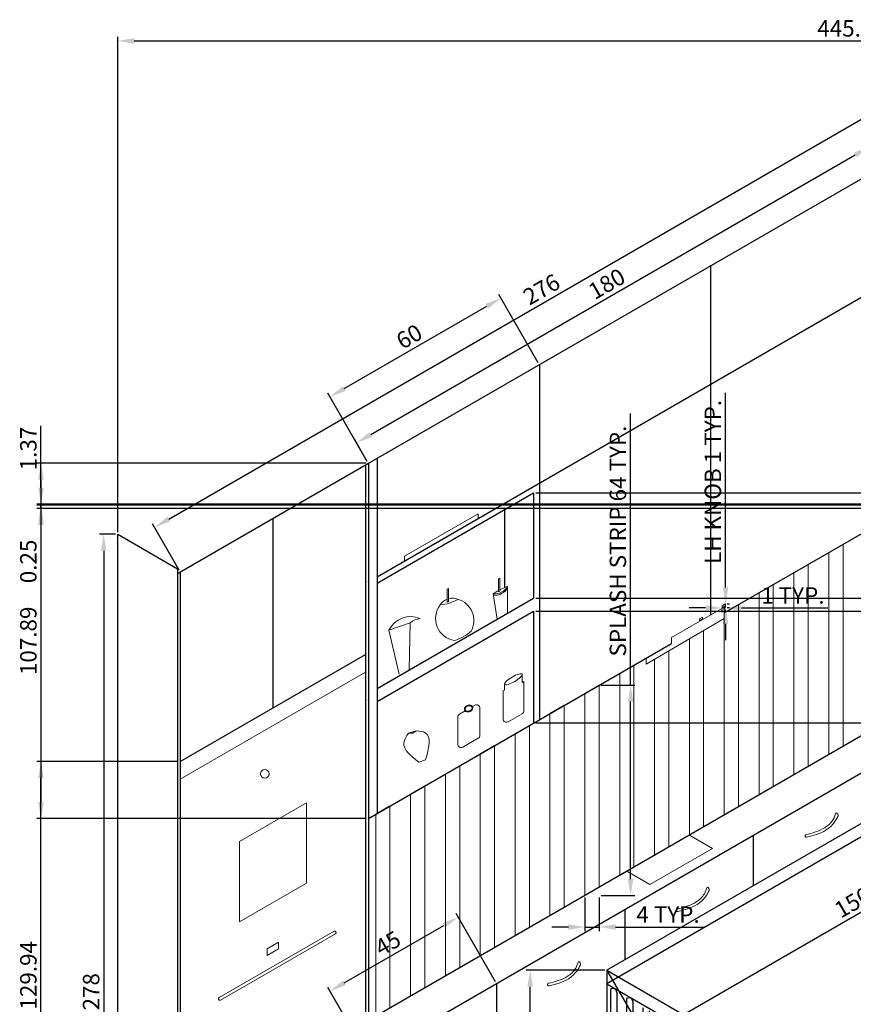
# Model space of a CAD drawing. Units: centimetres. Extents: x 2148 to 2649, y 4226 to 4785.
# Tile 2 of 6: x 2148 to 2402, y 4445 to 4744. Entities that reach past the tile are written whole.
import ezdxf

# ---------------------------------------------------------------- set-up
doc = ezdxf.new("R2010")
doc.units = ezdxf.units.CM
for name, color, linetype, lineweight in [('A-ANNO-DIMS', 63, 'Continuous', 18), ('A-ANNO-REFR', 8, 'Continuous', 13), ('A-EQPM', 30, 'Continuous', 18), ('A-FLOR-BSPL', 21, 'Continuous', 13), ('A-FLOR-CASE', 21, 'Continuous', 25), ('A-FLOR-CASE-HDW', 21, 'Continuous', 18), ('A-FLOR-CASE-TALL', 30, 'Continuous', 30), ('A-FLOR-CTOP', 21, 'Continuous', 25), ('A-FURN-ACCS', 21, 'Continuous', 13), ('TABLE', 30, 'Continuous', 25)]:
    doc.layers.add(name, color=color, linetype=linetype, lineweight=lineweight)
doc.styles.get("Standard").update_dxf_attribs({"font": 'arial.ttf'})
doc.dimstyles.new('ISO-25', dxfattribs={"dimtxt": 5, "dimasz": 5, "dimexe": 1.25, "dimexo": 0.625, "dimtad": 1, "dimdec": 1, "dimtxsty": 'Standard', "dimcen": 2.5, "dimadec": 0, "dimazin": 0, "dimtfac": 1, "dimtdec": 1, "dimtmove": 0, "dimatfit": 3, "dimfxl": 1, "dimarcsym": 0})

# ---------------------------------------------------------------- blocks, each defined once
blk = doc.blocks.new('*D1')
at = {"layer": 'A-ANNO-DIMS', "color": 0, "lineweight": -2, "transparency": 16777216}
for p, q in [((2409.99, 4699.79), (2406.08, 4706.55)), ((2255.15, 4617.96), (2402.38, 4702.96)), ((2254.1, 4609.79), (2250.2, 4616.55))]:
    blk.add_line(p, q, dxfattribs=at)
at = {"layer": 'A-ANNO-DIMS', "color": 0, "transparency": 16777216}
for points in [[(2401.96, 4703.69), (2402.8, 4702.24), (2406.71, 4705.46)], [(2254.74, 4618.69), (2255.57, 4617.24), (2250.82, 4615.46)]]:
    blk.add_solid(points, dxfattribs=at)
at = {"layer": 'Defpoints', "color": 0, "transparency": 16777216}
for p in [(2406.71, 4705.46), (2410.3, 4699.24), (2254.42, 4609.24)]:
    blk.add_point(p, dxfattribs=at)
at = {"layer": 'A-ANNO-DIMS', "color": 0, "transparency": 16777216, "insert": (2327.18, 4663.22), "char_height": 5, "attachment_point": 5, "rotation": 30}
blk.add_mtext('180', dxfattribs=at)
blk = doc.blocks.new('RECTANGLE')
for p, q in [((2256.66, 4502.65), (2260.99, 4505.15)), ((2256.66, 4502.65), (2256.66, 4441.26)), ((2260.99, 4443.76), (2260.99, 4505.15)), ((2256.66, 4441.26), (2260.99, 4443.76))]:
    blk.add_line(p, q)
blk = doc.blocks.new('*D4')
at = {"layer": 'A-ANNO-DIMS', "color": 0, "lineweight": -2, "transparency": 16777216}
for p, q in [((2177.63, 4587.69), (2172.75, 4587.69)), ((2174, 4582.69), (2174, 4314.69)), ((2177.63, 4309.69), (2172.75, 4309.69))]:
    blk.add_line(p, q, dxfattribs=at)
at = {"layer": 'A-ANNO-DIMS', "color": 0, "transparency": 16777216}
for points in [[(2173.16, 4582.69), (2174.83, 4582.69), (2174, 4587.69)], [(2173.16, 4314.69), (2174.83, 4314.69), (2174, 4309.69)]]:
    blk.add_solid(points, dxfattribs=at)
at = {"layer": 'Defpoints', "color": 0, "transparency": 16777216}
for p in [(2178.26, 4587.69), (2174, 4309.69), (2178.26, 4309.69)]:
    blk.add_point(p, dxfattribs=at)
at = {"layer": 'A-ANNO-DIMS', "color": 0, "transparency": 16777216, "insert": (2170.82, 4448.69), "char_height": 5, "attachment_point": 5, "rotation": 90}
blk.add_mtext('278', dxfattribs=at)
blk = doc.blocks.new('*D5')
at = {"layer": 'A-ANNO-DIMS', "color": 0, "lineweight": -2, "transparency": 16777216}
for p, q in [((2435.97, 4714.79), (2427.84, 4728.87)), ((2193.77, 4592.29), (2424.13, 4725.29)), ((2196.95, 4576.79), (2188.81, 4590.87))]:
    blk.add_line(p, q, dxfattribs=at)
at = {"layer": 'A-ANNO-DIMS', "color": 0, "transparency": 16777216}
for points in [[(2423.72, 4726.01), (2424.55, 4724.57), (2428.46, 4727.79)], [(2193.35, 4593.01), (2194.19, 4591.57), (2189.44, 4589.79)]]:
    blk.add_solid(points, dxfattribs=at)
at = {"layer": 'Defpoints', "color": 0, "transparency": 16777216}
for p in [(2428.46, 4727.79), (2436.28, 4714.24), (2197.26, 4576.24)]:
    blk.add_point(p, dxfattribs=at)
at = {"layer": 'A-ANNO-DIMS', "color": 0, "transparency": 16777216, "insert": (2307.36, 4661.54), "char_height": 5, "attachment_point": 5, "rotation": 30}
blk.add_mtext('276', dxfattribs=at)
blk = doc.blocks.new('T')
for p, q in [((2448.14, 4353.09), (2318.24, 4278.09)), ((2522.91, 4309.92), (2448.14, 4353.09)), ((2403.01, 4232.03), (2522.91, 4301.26)), ((2318.24, 4278.09), (2398.01, 4232.03))]:
    blk.add_line(p, q)
for centre, start, end in [((2520.41, 4305.59), 300, 60), ((2400.51, 4236.36), 240, 300)]:
    blk.add_arc(centre, 5, start, end)
blk = doc.blocks.new('FRUITS')
for centre in [(2416.61, 4474.09), (2427.91, 4474), (2437.55, 4475.46), (2421.39, 4472.47)]:
    blk.add_circle(centre, 1.88)
for centre, start, end in [((2425.68, 4477.15), 250.6785, 228.1131), ((2431.37, 4476.49), 347.1742, 260.6235), ((2420.14, 4474.94), 339.5983, 177.9649), ((2423.8, 4473.97), 252.9307, 170.9248), ((2432.9, 4474.21), 301.9934, 262.6603), ((2420.14, 4474.94), 208.8656, 254.0869)]:
    blk.add_arc(centre, 1.88, start, end)
for start_param, end_param in [(5.976427, 9.8373), (4.471607, 4.914134)]:
    blk.add_ellipse((2418.08, 4470.84), major_axis=(-2.82, 1), ratio=0.809593, start_param=start_param, end_param=end_param)
for points, knots in [([(2406.43, 4471.88), (2412.49, 4474.08), (2424.62, 4478.48), (2437.33, 4476.24), (2443.7, 4475.12)], [0, 0, 0, 0, 18.967698, 37.99902, 37.99902, 37.99902, 37.99902]), ([(2406.43, 4471.88), (2409.22, 4465.94), (2414.78, 4454.12), (2438.7, 4455.69), (2442.02, 4468.59), (2443.7, 4475.12)], [0, 0, 0, 0, 18.249558, 36.298645, 54.808813, 54.808813, 54.808813, 54.808813]), ([(2406.43, 4471.88), (2411.36, 4471.29), (2423.93, 4469.77), (2436.23, 4473.1), (2443.7, 4475.12)], [0, 0, 0, 0, 14.783083, 37.710843, 37.710843, 37.710843, 37.710843])]:
    blk.add_open_spline(points, degree=3, knots=knots)
blk = doc.blocks.new('TABLE 3')
for p, q in [((2534.09, 4482.72), (2534.09, 4425.1)), ((2529.29, 4472.97), (2529.29, 4424.6)), ((2531.69, 4473.13), (2531.69, 4424.8)), ((2531.69, 4473.13), (2531.69, 4424.8)), ((2523.55, 4469.66), (2523.55, 4424.61)), ((2525.96, 4471.05), (2525.96, 4423.89)), ((2525.96, 4469.82), (2525.96, 4423.89)), ((2529.29, 4471.74), (2529.29, 4424.6)), ((2520.23, 4467.74), (2520.23, 4430.04)), ((2520.23, 4466.51), (2520.23, 4430.04)), ((2523.55, 4468.43), (2523.55, 4424.61)), ((2514.5, 4464.43), (2514.5, 4434.64)), ((2517.82, 4466.35), (2517.82, 4432.4)), ((2517.82, 4465.12), (2517.82, 4432.4)), ((2508.76, 4461.12), (2508.76, 4432.32)), ((2512.09, 4463.04), (2512.09, 4434.39)), ((2512.09, 4461.81), (2512.09, 4434.39)), ((2514.5, 4463.2), (2514.5, 4434.64)), ((2503.03, 4457.81), (2503.03, 4427.36)), ((2506.35, 4459.73), (2506.35, 4430.48)), ((2506.35, 4458.5), (2506.35, 4430.48)), ((2326.91, 4455.22), (2326.91, 4314.1)), ((2497.3, 4454.5), (2497.3, 4419.33)), ((2500.62, 4456.42), (2500.62, 4424.52)), ((2500.62, 4455.19), (2500.62, 4424.52)), ((2503.03, 4456.58), (2503.03, 4427.36)), ((2494.89, 4453.11), (2494.89, 4413.65)), ((2494.89, 4451.88), (2494.89, 4413.65)), ((2497.3, 4453.27), (2497.3, 4419.33)), ((2328.01, 4449.42), (2328.01, 4314.3)), ((2329.93, 4448.55), (2329.93, 4313.58)), ((2489.16, 4449.8), (2489.16, 4412.9)), ((2489.16, 4448.57), (2489.16, 4412.9)), ((2491.57, 4451.19), (2491.57, 4413.39)), ((2491.57, 4449.96), (2491.57, 4413.39)), ((2332.9, 4446.6), (2332.9, 4311.48)), ((2334.82, 4445.73), (2334.82, 4310.75)), ((2483.42, 4446.49), (2483.42, 4412.26)), ((2485.83, 4447.88), (2485.83, 4412.44)), ((2485.83, 4446.65), (2485.83, 4412.44)), ((2337.79, 4443.77), (2337.79, 4308.66)), ((2339.71, 4442.9), (2339.71, 4307.93)), ((2480.1, 4443.34), (2480.1, 4410.27)), ((2480.1, 4443.34), (2480.1, 4410.27)), ((2483.42, 4445.26), (2483.42, 4412.26)), ((2342.68, 4440.95), (2342.68, 4305.83)), ((2344.61, 4440.08), (2344.61, 4305.11)), ((2474.37, 4440.03), (2474.37, 4418.94)), ((2477.69, 4441.95), (2477.69, 4415.46)), ((2477.69, 4441.95), (2477.69, 4415.46)), ((2347.58, 4438.12), (2347.58, 4303.01)), ((2349.5, 4437.25), (2349.5, 4302.28)), ((2468.64, 4436.72), (2468.64, 4419.49)), ((2468.64, 4436.72), (2468.64, 4419.49)), ((2352.47, 4435.3), (2352.47, 4300.18)), ((2354.39, 4434.43), (2354.39, 4299.46)), ((2466.23, 4435.33), (2466.23, 4418.06)), ((2466.23, 4435.33), (2466.23, 4418.06)), ((2357.36, 4432.47), (2357.36, 4297.36)), ((2359.28, 4431.6), (2359.28, 4296.63)), ((2460.49, 4432.02), (2460.49, 4413.4)), ((2460.49, 4432.02), (2460.49, 4413.4)), ((2462.9, 4433.41), (2462.9, 4415.61)), ((2462.9, 4433.41), (2462.9, 4415.61)), ((2362.25, 4429.65), (2362.25, 4294.53)), ((2364.18, 4428.78), (2364.18, 4293.81)), ((2454.76, 4428.71), (2454.76, 4405.82)), ((2457.17, 4430.1), (2457.17, 4409.54)), ((2457.17, 4430.1), (2457.17, 4409.54)), ((2367.15, 4426.82), (2367.15, 4291.71)), ((2369.07, 4425.95), (2369.07, 4290.98)), ((2449.03, 4425.4), (2449.03, 4290.41)), ((2451.44, 4426.79), (2451.44, 4291.8)), ((2372.04, 4424), (2372.04, 4288.88)), ((2373.96, 4423.13), (2373.96, 4288.16)), ((2443.3, 4422.09), (2443.3, 4287.1)), ((2445.7, 4423.48), (2445.7, 4288.49)), ((2376.93, 4421.17), (2376.93, 4286.06)), ((2378.85, 4420.3), (2378.85, 4285.33)), ((2437.56, 4418.78), (2437.56, 4283.79)), ((2439.97, 4420.17), (2439.97, 4285.18)), ((2381.82, 4418.35), (2381.82, 4283.23)), ((2383.75, 4417.48), (2383.75, 4282.51)), ((2434.24, 4416.86), (2434.24, 4281.87)), ((2386.72, 4415.52), (2386.72, 4280.41)), ((2388.64, 4414.65), (2388.64, 4279.68)), ((2391.61, 4412.7), (2391.61, 4277.58)), ((2428.51, 4413.55), (2428.51, 4278.56)), ((2431.83, 4415.47), (2431.83, 4280.48)), ((2393.53, 4411.83), (2393.53, 4276.86)), ((2396.5, 4409.88), (2396.5, 4274.76)), ((2422.77, 4410.24), (2422.77, 4275.25)), ((2426.1, 4412.16), (2426.1, 4277.17)), ((2398.42, 4409.01), (2398.42, 4274.03)), ((2400.52, 4408.63), (2400.52, 4271.6)), ((2417.84, 4408.63), (2417.84, 4271.6)), ((2420.37, 4408.85), (2420.37, 4273.86)), ((2460.49, 4392.27), (2460.49, 4323.14)), ((2503.03, 4391.9), (2503.03, 4330.42)), ((2462.9, 4390.64), (2462.9, 4321.75)), ((2500.62, 4390.56), (2500.62, 4329.03)), ((2512.09, 4390.5), (2512.09, 4334.07)), ((2523.55, 4388.81), (2523.55, 4340.69)), ((2525.96, 4389.23), (2525.96, 4342.08)), ((2534.09, 4391.22), (2534.09, 4381.5)), ((2466.23, 4388.14), (2466.23, 4319.83)), ((2468.64, 4386.14), (2468.64, 4318.44)), ((2491.57, 4386.54), (2491.57, 4323.8)), ((2494.89, 4387.83), (2494.89, 4325.72)), ((2520.23, 4388.33), (2520.23, 4338.77)), ((2477.69, 4383.14), (2477.69, 4315.79)), ((2480.1, 4383.51), (2480.1, 4317.18)), ((2483.42, 4384.17), (2483.42, 4319.1)), ((2485.83, 4384.76), (2485.83, 4320.49)), ((2534.09, 4384.82), (2534.09, 4341.83)), ((2529.29, 4341), (2529.29, 4336.74)), ((2525.96, 4339.08), (2525.96, 4334.83)), ((2518.06, 4329.46), (2529.88, 4336.29)), ((2520.23, 4335.77), (2520.23, 4331.52)), ((2523.55, 4337.69), (2523.55, 4333.43)), ((2512.09, 4331.07), (2512.09, 4326.82)), ((2508.53, 4323.96), (2515.55, 4328.01)), ((2500.62, 4323.12), (2500.62, 4322.24)), ((2503.03, 4324.51), (2503.03, 4321.59)), ((2494.89, 4319.81), (2494.89, 4316.89)), ((2503.09, 4320.82), (2506.45, 4322.76)), ((2460.49, 4317.23), (2460.49, 4297.03)), ((2475.33, 4304.79), (2496.19, 4316.83)), ((2491.57, 4317.89), (2491.57, 4314.97)), ((2498.19, 4317.99), (2500.49, 4319.32)), ((2326.91, 4314.1), (2406.68, 4268.04)), ((2462.9, 4315.84), (2462.9, 4298.42)), ((2466.23, 4313.92), (2466.23, 4300.34)), ((2485.83, 4314.58), (2485.83, 4311.66)), ((2489.16, 4316.5), (2489.16, 4313.58)), ((2468.64, 4312.53), (2468.64, 4301.73)), ((2480.1, 4311.27), (2480.1, 4308.35)), ((2483.42, 4313.19), (2483.42, 4310.27)), ((2477.69, 4309.88), (2477.69, 4306.96)), ((2455.96, 4293.61), (2473.25, 4303.59)), ((2411.68, 4268.04), (2454.39, 4292.7))]:
    blk.add_line(p, q)
for centre, radius, start, end in [((2530.67, 4472.12), 1.44, 44.5272, 195.4728), ((2524.94, 4468.81), 1.44, 44.5272, 195.4728), ((2519.2, 4465.5), 1.44, 44.5272, 195.4728), ((2513.47, 4462.19), 1.44, 44.5272, 195.4728), ((2507.74, 4458.88), 1.44, 44.5272, 195.4728), ((2502.01, 4455.57), 1.44, 44.5272, 195.4728), ((2496.27, 4452.26), 1.44, 44.5272, 195.4728), ((2490.54, 4448.95), 1.44, 44.5272, 195.4728), ((2484.81, 4445.64), 1.44, 44.5272, 195.4728), ((2479.08, 4442.33), 1.44, 44.5272, 195.4728), ((2473.34, 4439.02), 1.44, 44.5272, 195.4728), ((2467.61, 4435.71), 1.44, 44.5272, 195.4728), ((2461.88, 4432.4), 1.44, 44.5272, 195.4728), ((2456.15, 4429.09), 1.44, 44.5272, 195.4728), ((2450.41, 4425.78), 1.44, 44.5272, 195.4728), ((2444.68, 4422.47), 1.44, 44.5272, 195.4728), ((2438.95, 4419.16), 1.44, 44.5272, 195.4728), ((2433.22, 4415.85), 1.44, 44.5272, 195.4728), ((2427.48, 4412.55), 1.44, 44.5272, 195.4728), ((2421.75, 4409.24), 1.44, 44.5272, 195.4728), ((2529.09, 4341.6), 5, 304.2234, 331.1295), ((2524.24, 4335.03), 1.74, 246.8122, 353.1878), ((2529.97, 4338.34), 1.74, 246.8122, 267.0744), ((2518.5, 4331.72), 1.74, 255.6127, 353.1878), ((2512.77, 4328.41), 1.74, 246.8122, 353.1878), ((2501.31, 4321.79), 1.74, 331.6217, 353.1878), ((2495.57, 4318.48), 1.74, 246.8122, 290.8785), ((2329.13, 4314.36), 1.12, 182.9367, 315.698), ((2489.84, 4315.17), 1.74, 246.8122, 353.1878), ((2334.02, 4311.54), 1.12, 182.9367, 315.698), ((2484.11, 4311.86), 1.74, 246.8122, 353.1878), ((2338.91, 4308.71), 1.12, 182.9367, 315.698), ((2478.38, 4308.55), 1.74, 246.8122, 353.1878), ((2343.8, 4305.89), 1.12, 182.9367, 315.698), ((2348.7, 4303.06), 1.12, 182.9367, 315.698), ((2353.59, 4300.24), 1.12, 182.9367, 315.698), ((2466.91, 4301.93), 1.74, 246.8122, 353.1878), ((2358.48, 4297.41), 1.12, 182.9367, 315.698), ((2461.18, 4298.62), 1.74, 246.8122, 353.1878), ((2363.37, 4294.59), 1.12, 182.9367, 315.698), ((2455.45, 4295.31), 1.74, 287.3713, 353.1878), ((2368.27, 4291.77), 1.12, 182.9367, 315.698), ((2449.71, 4292.01), 1.74, 246.8122, 353.1878), ((2373.16, 4288.94), 1.12, 182.9367, 315.698), ((2443.98, 4288.7), 1.74, 246.8122, 353.1878), ((2378.05, 4286.12), 1.12, 182.9367, 315.698), ((2438.25, 4285.39), 1.74, 246.8122, 353.1878), ((2382.94, 4283.29), 1.12, 182.9367, 315.698), ((2432.51, 4282.08), 1.74, 246.8122, 353.1878), ((2387.84, 4280.47), 1.12, 182.9367, 315.698), ((2426.78, 4278.77), 1.74, 246.8122, 353.1878), ((2392.73, 4277.64), 1.12, 182.9367, 315.698), ((2421.05, 4275.46), 1.74, 246.8122, 353.1878), ((2397.62, 4274.82), 1.12, 182.9367, 315.698), ((2409.18, 4272.37), 5, 240, 300)]:
    blk.add_arc(centre, radius, start, end)
for name, p in [('T', (8.67, 177.13)), ('T', (8.67, 173.04)), ('FRUITS', (0, 0))]:
    blk.add_blockref(name, p)
blk = doc.blocks.new('PULL-BASE-BOW')
for centre, radius, start, end in [((9.29, 6.64), 0.774, 341.702, 83.222), ((0.41, 0.41), 0.414, 116.0189, 282.6641)]:
    blk.add_arc(centre, radius, start, end)
for points, knots in [([(0.23, 0.79), (2.23, 1.29), (5.42, 2.1), (8.53, 4.9), (9.15, 6.73), (9.38, 7.41)], [0, 0, 0, 0, 6.127515, 9.756066, 11.887711, 11.887711, 11.887711, 11.887711]), ([(0.5, 0.01), (2.55, 0.54), (5.72, 1.35), (8.78, 4.08), (9.68, 5.75), (10.03, 6.4)], [0, 0, 0, 0, 6.234589, 9.67204, 11.894402, 11.894402, 11.894402, 11.894402])]:
    blk.add_open_spline(points, degree=3, knots=knots)
blk = doc.blocks.new('KNOB-ISO-L')
for p, q in [((0, 0.53), (0.92, 1.06)), ((0, 0), (0, 0.53)), ((0, 0), (0.92, 0.53)), ((0.92, 1.06), (0.92, 0.53))]:
    blk.add_line(p, q)
blk = doc.blocks.new('*D20')
at = {"layer": 'A-ANNO-DIMS', "color": 0, "lineweight": -2, "transparency": 16777216}
for p, q in [((2334.1, 4541.83), (2334.1, 4624.41)), ((2325.14, 4541.83), (2335.35, 4541.83)), ((2334.1, 4482.94), (2334.1, 4536.83)), ((2325.14, 4477.94), (2335.35, 4477.94))]:
    blk.add_line(p, q, dxfattribs=at)
at = {"layer": 'A-ANNO-DIMS', "color": 0, "transparency": 16777216}
for points in [[(2333.27, 4536.83), (2334.94, 4536.83), (2334.1, 4541.83)], [(2333.27, 4482.94), (2334.94, 4482.94), (2334.1, 4477.94)]]:
    blk.add_solid(points, dxfattribs=at)
at = {"layer": 'Defpoints', "color": 0, "transparency": 16777216}
for p in [(2324.52, 4541.83), (2334.1, 4541.83), (2324.52, 4477.94)]:
    blk.add_point(p, dxfattribs=at)
at = {"layer": 'A-ANNO-DIMS', "color": 0, "transparency": 16777216, "insert": (2330.89, 4585.62), "char_height": 5, "attachment_point": 5, "rotation": 90}
blk.add_mtext('SPLASH STRIP 64 TYP.', dxfattribs=at)
blk = doc.blocks.new('*D21')
at = {"layer": 'A-ANNO-DIMS', "color": 0, "lineweight": -2, "transparency": 16777216}
for p, q in [((2320.19, 4477.31), (2320.19, 4467.1)), ((2324.52, 4477.31), (2324.52, 4467.1)), ((2315.19, 4468.35), (2310.19, 4468.35)), ((2320.19, 4468.35), (2324.52, 4468.35)), ((2329.52, 4468.35), (2356.42, 4468.35))]:
    blk.add_line(p, q, dxfattribs=at)
at = {"layer": 'A-ANNO-DIMS', "color": 0, "transparency": 16777216}
for points in [[(2315.19, 4469.19), (2315.19, 4467.52), (2320.19, 4468.35)], [(2329.52, 4469.19), (2329.52, 4467.52), (2324.52, 4468.35)]]:
    blk.add_solid(points, dxfattribs=at)
at = {"layer": 'Defpoints', "color": 0, "transparency": 16777216}
for p in [(2320.19, 4477.94), (2324.52, 4477.94), (2324.52, 4468.35)]:
    blk.add_point(p, dxfattribs=at)
at = {"layer": 'A-ANNO-DIMS', "color": 0, "transparency": 16777216, "insert": (2345.47, 4471.48), "char_height": 5, "attachment_point": 5}
blk.add_mtext('4 TYP.', dxfattribs=at)
blk = doc.blocks.new('*D24')
at = {"layer": 'A-ANNO-DIMS', "color": 0, "lineweight": -2, "transparency": 16777216}
for p, q in [((2362.95, 4571.52), (2362.95, 4630.61)), ((2362.95, 4565.46), (2362.95, 4566.52)), ((2363.42, 4566.52), (2364.2, 4566.52)), ((2363.42, 4565.46), (2364.2, 4565.46)), ((2362.95, 4560.46), (2362.95, 4555.46))]:
    blk.add_line(p, q, dxfattribs=at)
at = {"layer": 'A-ANNO-DIMS', "color": 0, "transparency": 16777216}
for points in [[(2362.12, 4571.52), (2363.78, 4571.52), (2362.95, 4566.52)], [(2362.12, 4560.46), (2363.78, 4560.46), (2362.95, 4565.46)]]:
    blk.add_solid(points, dxfattribs=at)
at = {"layer": 'Defpoints', "color": 0, "transparency": 16777216}
for p in [(2362.79, 4566.52), (2362.79, 4565.46), (2362.95, 4566.52)]:
    blk.add_point(p, dxfattribs=at)
at = {"layer": 'A-ANNO-DIMS', "color": 0, "transparency": 16777216, "insert": (2359.74, 4603.57), "char_height": 5, "attachment_point": 5, "rotation": 90}
blk.add_mtext('LH KNOB 1 TYP.', dxfattribs=at)
blk = doc.blocks.new('*D25')
at = {"layer": 'A-ANNO-DIMS', "color": 0, "lineweight": -2, "transparency": 16777216}
for p, q in [((2356.87, 4565.3), (2351.87, 4565.3)), ((2361.87, 4565.3), (2362.79, 4565.3)), ((2367.79, 4565.3), (2394.02, 4565.3)), ((2361.87, 4564.84), (2361.87, 4564.05)), ((2362.79, 4564.84), (2362.79, 4564.05))]:
    blk.add_line(p, q, dxfattribs=at)
at = {"layer": 'A-ANNO-DIMS', "color": 0, "transparency": 16777216}
for points in [[(2356.87, 4566.13), (2356.87, 4564.47), (2361.87, 4565.3)], [(2367.79, 4566.13), (2367.79, 4564.47), (2362.79, 4565.3)]]:
    blk.add_solid(points, dxfattribs=at)
at = {"layer": 'Defpoints', "color": 0, "transparency": 16777216}
for p in [(2361.87, 4565.46), (2362.79, 4565.46), (2362.79, 4565.3)]:
    blk.add_point(p, dxfattribs=at)
at = {"layer": 'A-ANNO-DIMS', "color": 0, "transparency": 16777216, "insert": (2383.41, 4568.44), "char_height": 5, "attachment_point": 5}
blk.add_mtext('1 TYP.', dxfattribs=at)
blk = doc.blocks.new('*D40')
at = {"layer": 'A-ANNO-DIMS', "color": 0, "lineweight": -2, "transparency": 16777216}
for p, q in [((2306.06, 4639.79), (2294.09, 4660.53)), ((2247.08, 4631.94), (2290.38, 4656.94)), ((2254.1, 4609.79), (2242.13, 4630.53))]:
    blk.add_line(p, q, dxfattribs=at)
at = {"layer": 'A-ANNO-DIMS', "color": 0, "transparency": 16777216}
for points in [[(2289.97, 4657.67), (2290.8, 4656.22), (2294.71, 4659.44)], [(2246.67, 4632.67), (2247.5, 4631.22), (2242.75, 4629.44)]]:
    blk.add_solid(points, dxfattribs=at)
at = {"layer": 'Defpoints', "color": 0, "transparency": 16777216}
for p in [(2294.71, 4659.44), (2306.38, 4639.24), (2254.42, 4609.24)]:
    blk.add_point(p, dxfattribs=at)
at = {"layer": 'A-ANNO-DIMS', "color": 0, "transparency": 16777216, "insert": (2267.15, 4647.2), "char_height": 5, "attachment_point": 5, "rotation": 30}
blk.add_mtext('60', dxfattribs=at)
blk = doc.blocks.new('*D41')
at = {"layer": 'A-ANNO-DIMS', "color": 0, "lineweight": -2, "transparency": 16777216}
for p, q in [((2253.79, 4609.24), (2153.68, 4609.24)), ((2154.93, 4604.24), (2154.93, 4506.36)), ((2253.79, 4501.36), (2153.68, 4501.36))]:
    blk.add_line(p, q, dxfattribs=at)
at = {"layer": 'A-ANNO-DIMS', "color": 0, "transparency": 16777216}
for points in [[(2154.1, 4604.24), (2155.77, 4604.24), (2154.93, 4609.24)], [(2154.1, 4506.36), (2155.77, 4506.36), (2154.93, 4501.36)]]:
    blk.add_solid(points, dxfattribs=at)
at = {"layer": 'Defpoints', "color": 0, "transparency": 16777216}
for p in [(2254.42, 4609.24), (2154.93, 4501.36), (2254.42, 4501.36)]:
    blk.add_point(p, dxfattribs=at)
at = {"layer": 'A-ANNO-DIMS', "color": 0, "transparency": 16777216, "insert": (2151.75, 4555.3), "char_height": 5, "attachment_point": 5, "rotation": 90}
blk.add_mtext('107.89', dxfattribs=at)
blk = doc.blocks.new('*D42')
at = {"layer": 'A-ANNO-DIMS', "color": 0, "lineweight": -2, "transparency": 16777216}
for p, q in [((2305.27, 4600.28), (2648.78, 4600.28)), ((2647.53, 4595.28), (2647.53, 4573.32)), ((2305.27, 4568.32), (2648.78, 4568.32))]:
    blk.add_line(p, q, dxfattribs=at)
at = {"layer": 'A-ANNO-DIMS', "color": 0, "transparency": 16777216}
for points in [[(2646.7, 4595.28), (2648.37, 4595.28), (2647.53, 4600.28)], [(2646.7, 4573.32), (2648.37, 4573.32), (2647.53, 4568.32)]]:
    blk.add_solid(points, dxfattribs=at)
at = {"layer": 'Defpoints', "color": 0, "transparency": 16777216}
for p in [(2304.65, 4600.28), (2304.65, 4568.32), (2647.53, 4568.32)]:
    blk.add_point(p, dxfattribs=at)
at = {"layer": 'A-ANNO-DIMS', "color": 0, "transparency": 16777216, "insert": (2644.35, 4584.3), "char_height": 5, "attachment_point": 5, "rotation": 90}
blk.add_mtext('31.96', dxfattribs=at)
blk = doc.blocks.new('*D43')
at = {"layer": 'A-ANNO-DIMS', "color": 0, "lineweight": -2, "transparency": 16777216}
for p, q in [((2647.53, 4573.32), (2647.53, 4578.32)), ((2305.27, 4568.32), (2648.78, 4568.32)), ((2647.53, 4568.32), (2647.53, 4564.32)), ((2305.27, 4564.32), (2648.78, 4564.32)), ((2647.53, 4559.32), (2647.53, 4549.61))]:
    blk.add_line(p, q, dxfattribs=at)
at = {"layer": 'A-ANNO-DIMS', "color": 0, "transparency": 16777216}
for points in [[(2646.7, 4573.32), (2648.37, 4573.32), (2647.53, 4568.32)], [(2646.7, 4559.32), (2648.37, 4559.32), (2647.53, 4564.32)]]:
    blk.add_solid(points, dxfattribs=at)
at = {"layer": 'Defpoints', "color": 0, "transparency": 16777216}
for p in [(2304.65, 4568.32), (2304.65, 4564.32), (2647.53, 4564.32)]:
    blk.add_point(p, dxfattribs=at)
at = {"layer": 'A-ANNO-DIMS', "color": 0, "transparency": 16777216, "insert": (2644.41, 4551.97), "char_height": 5, "attachment_point": 5, "rotation": 90}
blk.add_mtext('4', dxfattribs=at)
blk = doc.blocks.new('*D44')
at = {"layer": 'A-ANNO-DIMS', "color": 0, "lineweight": -2, "transparency": 16777216}
for p, q in [((2305.27, 4564.32), (2648.78, 4564.32)), ((2647.53, 4559.32), (2647.53, 4535.36)), ((2305.27, 4530.36), (2648.78, 4530.36))]:
    blk.add_line(p, q, dxfattribs=at)
at = {"layer": 'A-ANNO-DIMS', "color": 0, "transparency": 16777216}
for points in [[(2646.7, 4559.32), (2648.37, 4559.32), (2647.53, 4564.32)], [(2646.7, 4535.36), (2648.37, 4535.36), (2647.53, 4530.36)]]:
    blk.add_solid(points, dxfattribs=at)
at = {"layer": 'Defpoints', "color": 0, "transparency": 16777216}
for p in [(2304.65, 4564.32), (2304.65, 4530.36), (2647.53, 4530.36)]:
    blk.add_point(p, dxfattribs=at)
at = {"layer": 'A-ANNO-DIMS', "color": 0, "transparency": 16777216, "insert": (2644.35, 4547.34), "char_height": 5, "attachment_point": 5, "rotation": 90}
blk.add_mtext('33.96', dxfattribs=at)
blk = doc.blocks.new('*D46')
at = {"layer": 'A-ANNO-DIMS', "color": 0, "lineweight": -2, "transparency": 16777216}
for p, q in [((2154.93, 4601.82), (2154.93, 4606.82)), ((2471.05, 4596.82), (2153.68, 4596.82)), ((2471.05, 4596.57), (2153.68, 4596.57)), ((2154.93, 4596.82), (2154.93, 4596.57)), ((2154.93, 4591.57), (2154.93, 4572.29))]:
    blk.add_line(p, q, dxfattribs=at)
at = {"layer": 'A-ANNO-DIMS', "color": 0, "transparency": 16777216}
for points in [[(2154.1, 4601.82), (2155.77, 4601.82), (2154.93, 4596.82)], [(2154.1, 4591.57), (2155.77, 4591.57), (2154.93, 4596.57)]]:
    blk.add_solid(points, dxfattribs=at)
at = {"layer": 'Defpoints', "color": 0, "transparency": 16777216}
for p in [(2154.93, 4596.57), (2471.68, 4596.82), (2471.68, 4596.57)]:
    blk.add_point(p, dxfattribs=at)
at = {"layer": 'A-ANNO-DIMS', "color": 0, "transparency": 16777216, "insert": (2151.75, 4579.43), "char_height": 5, "attachment_point": 5, "rotation": 90}
blk.add_mtext('0.25', dxfattribs=at)
blk = doc.blocks.new('*D49')
at = {"layer": 'A-ANNO-DIMS', "color": 0, "lineweight": -2, "transparency": 16777216}
for p, q in [((2154.93, 4601.85), (2154.93, 4620.61)), ((2470.57, 4596.85), (2153.68, 4596.85)), ((2471.81, 4595.48), (2153.68, 4595.48)), ((2154.93, 4595.48), (2154.93, 4596.85)), ((2154.93, 4590.48), (2154.93, 4585.48))]:
    blk.add_line(p, q, dxfattribs=at)
at = {"layer": 'A-ANNO-DIMS', "color": 0, "transparency": 16777216}
for points in [[(2154.1, 4601.85), (2155.77, 4601.85), (2154.93, 4596.85)], [(2154.1, 4590.48), (2155.77, 4590.48), (2154.93, 4595.48)]]:
    blk.add_solid(points, dxfattribs=at)
at = {"layer": 'Defpoints', "color": 0, "transparency": 16777216}
for p in [(2154.93, 4596.85), (2471.19, 4596.85), (2472.44, 4595.48)]:
    blk.add_point(p, dxfattribs=at)
at = {"layer": 'A-ANNO-DIMS', "color": 0, "transparency": 16777216, "insert": (2151.75, 4613.73), "char_height": 5, "attachment_point": 5, "rotation": 90}
blk.add_mtext('1.37', dxfattribs=at)
blk = doc.blocks.new('*D50')
at = {"layer": 'A-ANNO-DIMS', "color": 0, "lineweight": -2, "transparency": 16777216}
for p, q in [((2178.26, 4588.31), (2178.26, 4738.82)), ((2624.21, 4606.37), (2624.21, 4738.82)), ((2183.26, 4737.57), (2619.21, 4737.57))]:
    blk.add_line(p, q, dxfattribs=at)
at = {"layer": 'A-ANNO-DIMS', "color": 0, "transparency": 16777216}
for points in [[(2183.26, 4738.4), (2183.26, 4736.74), (2178.26, 4737.57)], [(2619.21, 4738.4), (2619.21, 4736.74), (2624.21, 4737.57)]]:
    blk.add_solid(points, dxfattribs=at)
at = {"layer": 'Defpoints', "color": 0, "transparency": 16777216}
for p in [(2624.21, 4737.57), (2624.21, 4605.74), (2178.26, 4587.69)]:
    blk.add_point(p, dxfattribs=at)
at = {"layer": 'A-ANNO-DIMS', "color": 0, "transparency": 16777216, "insert": (2401.23, 4740.75), "char_height": 5, "attachment_point": 5}
blk.add_mtext('445.95', dxfattribs=at)
blk = doc.blocks.new('*D54')
at = {"layer": 'A-ANNO-DIMS', "color": 0, "lineweight": -2, "transparency": 16777216}
for p, q in [((2196.63, 4518.66), (2153.68, 4518.66)), ((2154.93, 4393.72), (2154.93, 4513.66)), ((2196.63, 4388.72), (2153.68, 4388.72))]:
    blk.add_line(p, q, dxfattribs=at)
at = {"layer": 'A-ANNO-DIMS', "color": 0, "transparency": 16777216}
for points in [[(2154.1, 4513.66), (2155.77, 4513.66), (2154.93, 4518.66)], [(2154.1, 4393.72), (2155.77, 4393.72), (2154.93, 4388.72)]]:
    blk.add_solid(points, dxfattribs=at)
at = {"layer": 'Defpoints', "color": 0, "transparency": 16777216}
for p in [(2154.93, 4518.66), (2197.26, 4518.66), (2197.26, 4388.72)]:
    blk.add_point(p, dxfattribs=at)
at = {"layer": 'A-ANNO-DIMS', "color": 0, "transparency": 16777216, "insert": (2151.75, 4453.69), "char_height": 5, "attachment_point": 5, "rotation": 90}
blk.add_mtext('129.94', dxfattribs=at)
blk = doc.blocks.new('*D56')
at = {"layer": 'A-ANNO-DIMS', "color": 0, "lineweight": -2, "transparency": 16777216}
for p, q in [((2326.29, 4455.22), (2302.34, 4455.22)), ((2303.59, 4319.1), (2303.59, 4450.22)), ((2326.29, 4314.1), (2302.34, 4314.1))]:
    blk.add_line(p, q, dxfattribs=at)
at = {"layer": 'A-ANNO-DIMS', "color": 0, "transparency": 16777216}
for points in [[(2302.75, 4450.22), (2304.42, 4450.22), (2303.59, 4455.22)], [(2302.75, 4319.1), (2304.42, 4319.1), (2303.59, 4314.1)]]:
    blk.add_solid(points, dxfattribs=at)
at = {"layer": 'Defpoints', "color": 0, "transparency": 16777216}
for p in [(2303.59, 4455.22), (2326.91, 4455.22), (2326.91, 4314.1)]:
    blk.add_point(p, dxfattribs=at)
at = {"layer": 'A-ANNO-DIMS', "color": 0, "transparency": 16777216, "insert": (2300.45, 4384.66), "char_height": 5, "attachment_point": 5, "rotation": 90}
blk.add_mtext('141.12', dxfattribs=at)
blk = doc.blocks.new('*D58')
at = {"layer": 'A-ANNO-DIMS', "color": 0, "lineweight": -2, "transparency": 16777216}
for p, q in [((2457.13, 4529.68), (2469.1, 4508.94)), ((2464.15, 4507.52), (2342.9, 4437.52)), ((2327.22, 4454.68), (2339.2, 4433.94))]:
    blk.add_line(p, q, dxfattribs=at)
at = {"layer": 'A-ANNO-DIMS', "color": 0, "transparency": 16777216}
for points in [[(2463.73, 4508.25), (2464.56, 4506.8), (2468.48, 4510.02)], [(2342.49, 4438.25), (2343.32, 4436.8), (2338.57, 4435.02)]]:
    blk.add_solid(points, dxfattribs=at)
at = {"layer": 'Defpoints', "color": 0, "transparency": 16777216}
for p in [(2456.81, 4530.22), (2326.91, 4455.22), (2338.57, 4435.02)]:
    blk.add_point(p, dxfattribs=at)
at = {"layer": 'A-ANNO-DIMS', "color": 0, "transparency": 16777216, "insert": (2401.94, 4475.28), "char_height": 5, "attachment_point": 5, "rotation": 30}
blk.add_mtext('150', dxfattribs=at)
blk = doc.blocks.new('*D66')
at = {"layer": 'A-ANNO-DIMS', "color": 0, "lineweight": -2, "transparency": 16777216}
for p, q in [((2293.07, 4451.7), (2281.1, 4472.44)), ((2247.08, 4451.36), (2277.39, 4468.86)), ((2254.1, 4429.2), (2242.13, 4449.94))]:
    blk.add_line(p, q, dxfattribs=at)
at = {"layer": 'A-ANNO-DIMS', "color": 0, "transparency": 16777216}
for points in [[(2276.98, 4469.58), (2277.81, 4468.14), (2281.72, 4471.36)], [(2246.67, 4452.08), (2247.5, 4450.64), (2242.75, 4448.86)]]:
    blk.add_solid(points, dxfattribs=at)
at = {"layer": 'Defpoints', "color": 0, "transparency": 16777216}
for p in [(2281.72, 4471.36), (2293.39, 4451.16), (2254.42, 4428.66)]:
    blk.add_point(p, dxfattribs=at)
at = {"layer": 'A-ANNO-DIMS', "color": 0, "transparency": 16777216, "insert": (2260.66, 4462.85), "char_height": 5, "attachment_point": 5, "rotation": 30}
blk.add_mtext('45', dxfattribs=at)

msp = doc.modelspace()

# ---------------------------------------------------------------- linework, layer by layer
at = {"layer": 'A-ANNO-REFR'}
for p in [(2358.3389, 4669.2447), (2306.3774, 4639.2447), (2254.4158, 4573.2822), (2254.4158, 4537.3196)]:
    msp.add_point(p, dxfattribs=at)
at = {"layer": 'A-EQPM'}
for p, q in [((2362.545, 4565.5444), (2346.4954, 4556.2782)), ((2362.545, 4562.0832), (2362.545, 4565.5444)), ((2338.8155, 4548.1884), (2362.545, 4562.0832)), ((2346.4954, 4556.2782), (2346.4954, 4554.5191)), ((2338.8155, 4550.0851), (2338.8155, 4548.1884)), ((2197.2581, 4513.2764), (2253.5498, 4545.7764)), ((2197.2581, 4513.2764), (2197.2581, 4388.7152)), ((2215.2302, 4494.3536), (2235.5778, 4506.1013)), ((2235.5778, 4506.1013), (2235.5778, 4481.6511)), ((2359.0306, 4492.2441), (2352.0006, 4496.3028)), ((2215.2302, 4469.9034), (2215.2302, 4494.3536)), ((2339.9737, 4481.2415), (2359.0306, 4492.2441)), ((2332.9437, 4485.3003), (2339.9737, 4481.2415)), ((2235.5778, 4481.6511), (2215.2302, 4469.9034)), ((2243.9913, 4467.0679), (2209.0748, 4446.9088)), ((2244.4244, 4466.3179), (2209.5078, 4446.1588)), ((2223.7008, 4461.7456), (2227.1623, 4463.7441)), ((2227.1623, 4463.7441), (2227.1623, 4461.7583)), ((2227.1623, 4461.7583), (2223.7008, 4459.7075)), ((2223.7008, 4459.7075), (2223.7008, 4461.7456))]:
    msp.add_line(p, q, dxfattribs=at)
msp.add_circle((2222.9447, 4514.8994), 1.2905, dxfattribs=at)
for centre, start, end in [((2244.2078, 4466.6929), 300, 120), ((2209.2913, 4446.5338), 120, 300)]:
    msp.add_arc(centre, 0.433, start, end, dxfattribs=at)
at = {"layer": 'A-FLOR-BSPL'}
for p, q in [((2356.2863, 4498.7772), (2356.2863, 4558.4184)), ((2351.9562, 4555.8829), (2351.9562, 4496.2772)), ((2345.6975, 4492.6638), (2345.6975, 4552.2182)), ((2341.3674, 4549.6827), (2341.3674, 4490.1638)), ((2351.9562, 4496.2772), (2356.2863, 4498.7772)), ((2341.3674, 4490.1638), (2345.6975, 4492.6638))]:
    msp.add_line(p, q, dxfattribs=at)
at = {"layer": 'A-FLOR-CASE'}
for p, q in [((2196.3921, 4575.7447), (2436.2812, 4714.2447)), ((2257.0504, 4574.8032), (2436.2812, 4678.2822)), ((2358.3389, 4669.2447), (2358.3389, 4563.1161)), ((2306.3774, 4639.2447), (2306.3774, 4531.357)), ((2257.0504, 4610.7658), (2257.0504, 4502.878)), ((2254.4158, 4609.2447), (2254.4158, 4342.0267)), ((2257.0504, 4572.8032), (2304.6453, 4600.2822)), ((2304.6453, 4600.2822), (2304.6453, 4568.3196)), ((2295.836, 4571.4862), (2295.836, 4595.1961)), ((2362.545, 4563.7854), (2410.3004, 4591.357)), ((2257.0504, 4540.8406), (2304.6453, 4568.3196)), ((2257.0504, 4536.8406), (2304.6453, 4564.3196)), ((2304.6453, 4564.3196), (2304.6453, 4530.357)), ((2254.4158, 4501.357), (2346.4954, 4554.5191)), ((2371.3293, 4496.1569), (2371.3293, 4480.8687)), ((2332.3581, 4473.6569), (2332.3581, 4458.3687)), ((2293.387, 4451.1569), (2293.387, 4364.5267))]:
    msp.add_line(p, q, dxfattribs=at)
at = {"layer": 'A-FLOR-CASE-HDW'}
for p, q in [((2265.4463, 4581.0026), (2287.7892, 4593.9023)), ((2287.7892, 4593.9023), (2287.7892, 4592.5503)), ((2265.4463, 4579.6506), (2265.4463, 4581.0026))]:
    msp.add_line(p, q, dxfattribs=at)
at = {"layer": 'A-FLOR-CASE-TALL'}
for p, q in [((2196.3921, 4575.7447), (2254.4158, 4609.2447)), ((2253.5498, 4608.7447), (2253.5498, 4331.2152)), ((2225.404, 4592.4947), (2225.404, 4534.906)), ((2178.2568, 4309.6856), (2178.2568, 4587.6856)), ((2178.2568, 4587.6856), (2196.3921, 4577.2152)), ((2196.3921, 4577.2152), (2196.3921, 4299.2152)), ((2197.2581, 4576.2447), (2197.2581, 4298.7152)), ((2197.2581, 4518.656), (2253.5498, 4551.156))]:
    msp.add_line(p, q, dxfattribs=at)
at = {"layer": 'A-FLOR-CTOP'}
for p, q in [((2410.3004, 4529.9623), (2254.4158, 4439.9623)), ((2410.3004, 4518.6569), (2254.4158, 4428.6569))]:
    msp.add_line(p, q, dxfattribs=at)
at = {"layer": 'A-FURN-ACCS'}
for p, q in [((2293.9783, 4574.1119), (2294.3493, 4574.3261)), ((2293.9783, 4570.2419), (2293.9783, 4574.1119)), ((2294.3493, 4574.3261), (2294.3493, 4570.4362)), ((2278.4036, 4570.9647), (2278.7746, 4571.1789)), ((2278.7746, 4571.1789), (2278.7746, 4567.289)), ((2296.7266, 4563.7477), (2296.7363, 4571.8625)), ((2278.4036, 4567.0947), (2278.4036, 4570.9647)), ((2293.5776, 4561.9296), (2292.3238, 4569.6255)), ((2260.6703, 4558.5519), (2267.1641, 4560.7735)), ((2267.1641, 4560.7735), (2266.8117, 4546.4763)), ((2263.8269, 4545.1447), (2260.6703, 4558.5519)), ((2301.1736, 4545.0733), (2301.1457, 4542.6455)), ((2295.8288, 4542.1033), (2295.8288, 4540.3333)), ((2301.1457, 4542.6455), (2301.6648, 4542.9452)), ((2301.6648, 4542.9452), (2301.6648, 4534.0206)), ((2295.8288, 4540.3333), (2295.3807, 4540.0746)), ((2295.3807, 4540.0746), (2295.3807, 4531.5471)), ((2286.0768, 4535.3098), (2286.8026, 4535.7288)), ((2282.1085, 4533.0186), (2283.8157, 4534.0043)), ((2288.3026, 4534.8628), (2288.3026, 4526.5895)), ((2296.8807, 4530.6811), (2301.1648, 4533.1545)), ((2281.6085, 4523.8793), (2281.6085, 4532.1526)), ((2266.6369, 4527.2937), (2268.9609, 4527.9963)), ((2287.8026, 4525.7235), (2283.1085, 4523.0133)), ((2269.7796, 4518.469), (2271.7939, 4519.1039))]:
    msp.add_line(p, q, dxfattribs=at)
for centre, radius, start, end in [((2292.8972, 4573.9649), 4.3771, 262.473031, 331.293661), ((2292.8972, 4573.5305), 4.3771, 263.425622, 331.293661), ((2306.7394, 4546.6608), 27.1143, 111.649138, 117.190829), ((2279.9561, 4563.8868), 4.3695, 66.774754, 105.688123), ((2306.7394, 4546.6608), 27.1143, 118.075847, 122.117554), ((2294.0332, 4570.5886), 0.351, 261.00406, 334.262617), ((2281.544, 4562.0876), 6.7053, 142.079886, 261.593641), ((2279.9561, 4563.8868), 4.3695, 110.81286, 147.905225), ((2274.8602, 4580.2079), 14.0687, 275.687311, 298.992669), ((2278.4584, 4567.4414), 0.351, 261.00406, 334.262617), ((2279.7442, 4561.4579), 6.7286, 331.130686, 73.286694), ((2267.2216, 4555.4107), 7.2654, 66.238708, 154.383269), ((2270.5972, 4556.9152), 5.1645, 94.978817, 131.66298), ((2277.5247, 4567.0981), 12.0338, 284.627881, 312.3835), ((2287.3026, 4534.8628), 1, 0, 120), ((2282.6085, 4532.1526), 1, 120, 180), ((2300.6648, 4534.0206), 1, 300, 0), ((2296.3807, 4531.5471), 1, 180, 300), ((2267.2355, 4529.4828), 2.2774, 254.390852, 319.253158), ((2287.3026, 4526.5895), 1, 300, 0), ((2282.6085, 4523.8793), 1, 180, 300)]:
    msp.add_arc(centre, radius, start, end, dxfattribs=at)
for centre, major_axis, ratio in [((2298.4872, 4543.6381), (2.6585, 1.5349), 0.25334948), ((2284.884, 4534.7498), (-1.0196, -0.4599), 0.71911236)]:
    msp.add_ellipse(centre, major_axis=major_axis, ratio=ratio, start_param=-1.57079633, end_param=4.71238898, dxfattribs=at)
for points, knots in [([(2284.471, 4535.6654), (2284.322, 4535.5981), (2284.1824, 4535.51), (2283.8758, 4535.2464), (2283.7335, 4535.0492), (2283.6032, 4534.6603), (2283.5948, 4534.472), (2283.6993, 4534.1296), (2283.8122, 4533.9797), (2284.1108, 4533.7705), (2284.2945, 4533.7093), (2284.6844, 4533.6719), (2284.8911, 4533.6955), (2285.4244, 4533.8585), (2285.734, 4534.0677), (2286.0609, 4534.5085), (2286.1425, 4534.7086), (2286.1663, 4535.1111), (2286.1038, 4535.3121), (2285.8516, 4535.6209), (2285.6675, 4535.727), (2285.2561, 4535.8291), (2285.0277, 4535.8267), (2284.6908, 4535.7514), (2284.5785, 4535.7138), (2284.471, 4535.6654)], [-1.57079633, -1.57079633, -1.57079633, -1.57079633, -1.18223207, -1.18223207, -0.58757548, -0.58757548, -0.09197206, -0.09197206, 0.40363136, 0.40363136, 0.89923477, 0.89923477, 1.39483819, 1.39483819, 2.23085544, 2.23085544, 2.78120121, 2.78120121, 3.33154698, 3.33154698, 3.88189275, 3.88189275, 4.43223853, 4.43223853, 4.71238898, 4.71238898, 4.71238898, 4.71238898]), ([(2266.6369, 4527.2937), (2265.9763, 4526.2779), (2263.8644, 4522.9939), (2267.3626, 4520.3179), (2269.7796, 4518.469)], [0.05033714, 0.05033714, 0.05033714, 0.05033714, 3.36690948, 10.78197101, 10.78197101, 10.78197101, 10.78197101]), ([(2268.9609, 4527.9963), (2269.9883, 4527.8823), (2274.0472, 4527.4322), (2272.7666, 4522.6722), (2271.7939, 4519.1039)], [0, 0, 0, 0, 2.80893941, 11.09695906, 11.09695906, 11.09695906, 11.09695906])]:
    msp.add_open_spline(points, degree=3, knots=knots, dxfattribs=at)
at = {"layer": 'TABLE'}
for centre in [(2328.7386, 4448.4782), (2333.631, 4445.6536)]:
    msp.add_arc(centre, 1.1926, 3.466055, 127.837068, dxfattribs=at)

# ---------------------------------------------------------------- block references
at = {"layer": 'A-FLOR-BSPL'}
for p in [(137.6542, 79.4747), (127.0654, 73.3612), (116.4766, 67.2478), (105.8878, 61.1344), (74.1215, 42.7941), (63.5327, 36.6806), (52.9439, 30.5672), (42.3551, 24.4537), (31.7663, 18.3403), (21.1776, 12.2269), (10.5888, 6.1134), (0, 0)]:
    msp.add_blockref('RECTANGLE', p, dxfattribs=at)
at = {"layer": 'A-FLOR-CASE-HDW'}
for name, p in [('KNOB-ISO-L', (2361.8744, 4565.4603)), ('KNOB-ISO-L', (2354.9903, 4561.4857)), ('PULL-BASE-BOW', (2387.0958, 4495.6294)), ('PULL-BASE-BOW', (2347.9533, 4473.0304)), ('PULL-BASE-BOW', (2308.8563, 4450.4578))]:
    msp.add_blockref(name, p, dxfattribs=at)
at = {"layer": 'TABLE'}
msp.add_blockref('TABLE 3', (0, 0), dxfattribs=at)

# ---------------------------------------------------------------- dimensions: what is measured, and where the dimension line sits
at = {"layer": 'A-ANNO-DIMS'}
dim = msp.add_linear_dim(base=(2624.2087, 4737.5697), p1=(2178.2568, 4587.6856), p2=(2624.2087, 4605.7447), dimstyle='ISO-25', override={"dimdec": 2, "dimlfac": 1, "dimrnd": 0, "dimzin": 0, "dimdsep": 46, "dimlunit": 2}, dxfattribs=at)
dim.commit()
dim.dimension.update_dxf_attribs({"geometry": '*D50', "text_midpoint": (2401.2328, 4740.7476)})
for p1, p2, distance, picture, middle in [((2197.2581, 4576.2447), (2436.2812, 4714.2447), 15.6376, '*D5', (2307.3619, 4661.5394)), ((2254.4158, 4609.2447), (2410.3004, 4699.2447), 7.1825, '*D1', (2327.1779, 4663.217)), ((2178.2568, 4587.6856), (2178.2568, 4309.6856), -4.2595, '*D4', (2170.8194, 4448.6856))]:
    dim = msp.add_aligned_dim(p1=p1, p2=p2, distance=distance, dimstyle='ISO-25', override={"dimclrd": 0, "dimclre": 0, "dimclrt": 0}, dxfattribs=at)
    dim.commit()
    dim.dimension.update_dxf_attribs({"geometry": picture, "text_midpoint": middle})
for base, p1, p2, angle, override, picture, middle in [((2294.7148, 4659.4448), (2254.4158, 4609.2447), (2306.3774, 4639.2447), 30, {"dimdec": 0, "dimlfac": 1, "dimrnd": 0, "dimzin": 0, "dimdsep": 46, "dimlunit": 2}, '*D40', (2267.1452, 4647.1969)), ((2154.9318, 4596.8477), (2472.4377, 4595.482), (2471.1914, 4596.8477), 90, {"dimdec": 2, "dimlfac": 1, "dimrnd": 0, "dimzin": 0, "dimdsep": 46, "dimlunit": 2}, '*D49', (2151.7523, 4613.7312)), ((2154.9318, 4501.357), (2254.4158, 4609.2447), (2254.4158, 4501.357), 90, {"dimdec": 2, "dimlfac": 1, "dimrnd": 0, "dimzin": 0, "dimdsep": 46, "dimlunit": 2}, '*D41', (2151.754, 4555.3009)), ((2154.9318, 4596.5668), (2471.6779, 4596.8213), (2471.6779, 4596.5668), 90, {"dimdec": 2, "dimlfac": 1, "dimrnd": 0, "dimzin": 0, "dimdsep": 46, "dimlunit": 2}, '*D46', (2151.754, 4579.4292)), ((2647.5337, 4568.3196), (2304.6453, 4600.2822), (2304.6453, 4568.3196), 90, {"dimdec": 2, "dimlfac": 1, "dimrnd": 0, "dimzin": 0, "dimdsep": 46, "dimlunit": 2}, '*D42', (2644.3541, 4584.3009)), ((2647.5337, 4564.3196), (2304.6453, 4568.3196), (2304.6453, 4564.3196), 90, {"dimdec": 0, "dimlfac": 1, "dimrnd": 0, "dimzin": 0, "dimdsep": 46, "dimlunit": 2}, '*D43', (2644.4087, 4551.9654)), ((2647.5337, 4530.357), (2304.6453, 4564.3196), (2304.6453, 4530.357), 90, {"dimdec": 2, "dimlfac": 1, "dimrnd": 0, "dimzin": 0, "dimdsep": 46, "dimlunit": 2}, '*D44', (2644.3541, 4547.3383)), ((2338.573, 4435.0235), (2456.8143, 4530.2236), (2326.9105, 4455.2236), 210, {"dimdec": 0, "dimlfac": 1, "dimrnd": 0, "dimzin": 0, "dimdsep": 46, "dimlunit": 2}, '*D58', (2401.936, 4475.2756)), ((2154.9318, 4518.656), (2197.2581, 4388.7152), (2197.2581, 4518.656), 90, {"dimdec": 2, "dimlfac": 1, "dimrnd": 0, "dimzin": 0, "dimdsep": 46, "dimlunit": 2}, '*D54', (2151.754, 4453.6856)), ((2281.7245, 4471.3569), (2254.4158, 4428.6569), (2293.387, 4451.1569), 30, {"dimdec": 0, "dimlfac": 1, "dimrnd": 0, "dimzin": 0, "dimdsep": 46, "dimlunit": 2}, '*D66', (2260.6551, 4462.8502)), ((2303.5855, 4455.2236), (2326.9105, 4314.0996), (2326.9105, 4455.2236), 90, {"dimdec": 2, "dimlfac": 1, "dimrnd": 0, "dimzin": 0, "dimdsep": 46, "dimlunit": 2}, '*D56', (2300.4503, 4384.6616))]:
    dim = msp.add_linear_dim(base=base, p1=p1, p2=p2, angle=angle, dimstyle='ISO-25', override=override, dxfattribs=at)
    dim.commit()
    dim.dimension.update_dxf_attribs({"geometry": picture, "text_midpoint": middle})
for base, p1, p2, text, picture, middle in [((2362.951, 4566.5217), (2362.7919, 4565.4606), (2362.7919, 4566.5217), 'LH KNOB <> TYP.', '*D24', (2359.7391, 4603.5655)), ((2334.1042, 4541.8316), (2324.5199, 4477.9369), (2324.5199, 4541.8316), 'SPLASH STRIP <> TYP.', '*D20', (2330.8939, 4585.6217))]:
    dim = msp.add_linear_dim(base=base, p1=p1, p2=p2, angle=90, text=text, dimstyle='ISO-25', override={"dimdec": 0, "dimlfac": 1, "dimrnd": 0, "dimzin": 0, "dimdsep": 46, "dimlunit": 2}, dxfattribs=at)
    dim.commit()
    dim.dimension.update_dxf_attribs({"geometry": picture, "text_midpoint": middle})
for base, p1, p2, picture, middle in [((2362.7919, 4565.3014), (2361.8742, 4565.4606), (2362.7919, 4565.4606), '*D25', (2383.4083, 4568.4383)), ((2324.5199, 4468.3527), (2320.1898, 4477.9369), (2324.5199, 4477.9369), '*D21', (2345.4724, 4471.4794))]:
    dim = msp.add_linear_dim(base=base, p1=p1, p2=p2, text='<> TYP.', dimstyle='ISO-25', override={"dimdec": 0, "dimlfac": 1, "dimrnd": 0, "dimzin": 0, "dimdsep": 46, "dimlunit": 2}, dxfattribs=at)
    dim.commit()
    dim.dimension.update_dxf_attribs({"geometry": picture, "text_midpoint": middle})

doc.saveas('drawing.dxf')
